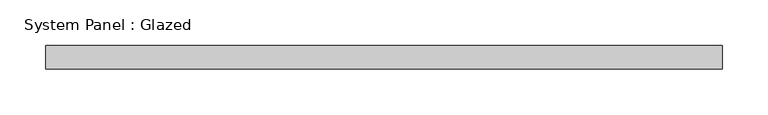
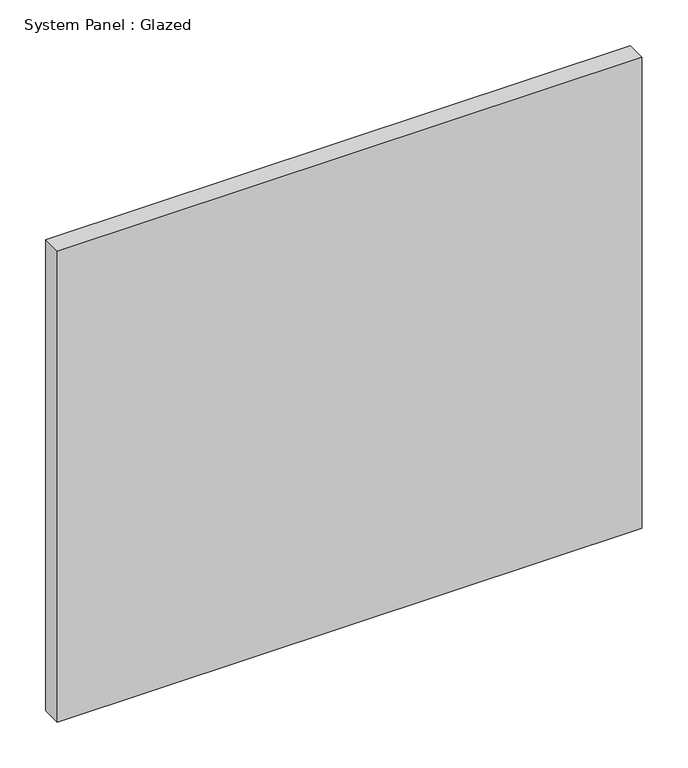
"""IFC4 building model written with IfcOpenShell, lengths in millimetres: plate geometry, System Panel : Glazed."""

from ifc_helpers import new_model, si_unit, origin, origin_with_axes, place, context, project, spatial, polyline, outline, extrude, source, transform, mapped, element, save


def system_panel_glazed_c1eeadb6(model_context):
    return source(origin(), model_context, "Body", "SweptSolid", [
        extrude(outline(polyline([(368.2890615, 19.05), (-368.2890615, 19.05), (-368.2890615, 44.45), (368.2890615, 44.45), (368.2890615, 19.05)])), origin_with_axes(), (0.0, 0.0, 1.0), 627.1281505),
    ])


if __name__ == "__main__":
    model = new_model("IFC4")
    model_context = context("Model", 3, world=origin())
    ifc_project = project(units=[si_unit("LENGTHUNIT", "METRE", prefix="MILLI")], contexts=[model_context])
    site = spatial("IfcSite", under=ifc_project)
    building = spatial("IfcBuilding", under=site)
    placement = place(None, origin())
    system_panel_glazed_shape = system_panel_glazed_c1eeadb6(model_context)
    element("IfcPlate", 1, ObjectType="System Panel : Glazed", at=placement, inside=building, context=model_context, shape_type="MappedRepresentation", body=[
        mapped(system_panel_glazed_shape, transform((0.0, 0.0, 0.0), x_axis=(1.0, 0.0, 0.0), y_axis=(0.0, 1.0, 0.0), z_axis=(0.0, 0.0, 1.0))),
    ])
    save(model, "model.ifc")

# Revit data of these elements
# Type "System Panel : Glazed"
#   Construction Type Id = "GSP4R"
#   Analytic Construction = "1/8 in Pilkington single glazing"
#   Visual Light Transmittance = 0.9
#   Solar Heat Gain Coefficient = 0.86
#   Heat Transfer Coefficient (U) = 1.18115 BTU/(h·ft²·°F)
#   Define Thermal Properties by = 1
# Element 1 (IfcPlate, "System Panel : Glazed")
#   Materials on its faces: "Glass"
# Materials
#   "Glass": class "Glass", colour RGB 0 128 192, transparency 0.75, Description = "Soda Lime Glass", Cost = 0
